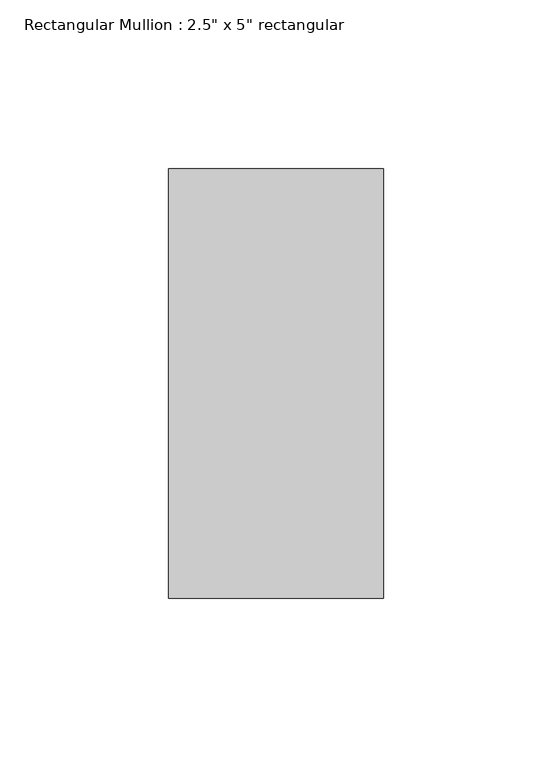
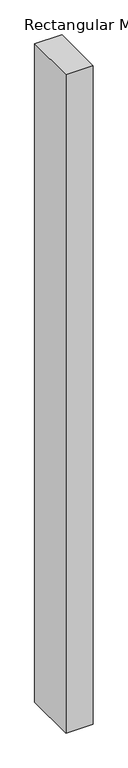
"""IFC4 building model written with IfcOpenShell, lengths in millimetres: member geometry."""

from ifc_helpers import new_model, si_unit, frame, origin, place, context, project, spatial, polyline, outline, extrude, source, transform, mapped, element, save


def member_87e6f62d(model_context):
    return source(origin(), model_context, "Body", "SweptSolid", [
        extrude(outline(polyline([(0.0, 63.5), (0.0, -63.5), (-63.5, -63.5), (-63.5, 63.5), (0.0, 63.5)])), frame((0.0, 0.0, -1630.7489674), z_axis=(0.0, 0.0, 1.0), x_axis=(1.0, 0.0, 0.0)), (0.0, 0.0, 1.0), 1630.7489674),
    ])


if __name__ == "__main__":
    model = new_model("IFC4")
    model_context = context("Model", 3, world=origin())
    ifc_project = project(units=[si_unit("LENGTHUNIT", "METRE", prefix="MILLI")], contexts=[model_context])
    site = spatial("IfcSite", under=ifc_project)
    building = spatial("IfcBuilding", under=site)
    placement = place(None, origin())
    member_shape = member_87e6f62d(model_context)
    element("IfcMember", 1, ObjectType="Rectangular Mullion : 2.5\" x 5\" rectangular", at=placement, inside=building, context=model_context, shape_type="MappedRepresentation", body=[
        mapped(member_shape, transform((0.0, 0.0, 0.0), x_axis=(1.0, 0.0, 0.0), y_axis=(0.0, 1.0, 0.0), z_axis=(0.0, 0.0, 1.0))),
    ])
    save(model, "model.ifc")

# Revit data of these elements
# Type "Rectangular Mullion : 2.5\" x 5\" rectangular"
#   built-in parameter 1007304 = 0.416667 (stored number, unit not read)
#   built-in parameter 1007301 = 0.104167 (stored number, unit not read)
#   built-in parameter 1007300 = 0.104167 (stored number, unit not read)
# Element 1 (IfcMember, "Rectangular Mullion : 2.5\" x 5\" rectangular")
#   Materials on its faces: "Aluminum"
# Materials
#   "Aluminum": class "Metal", colour RGB 247 247 247, transparency 0, Description = "Aluminum 6061", Cost = 0
